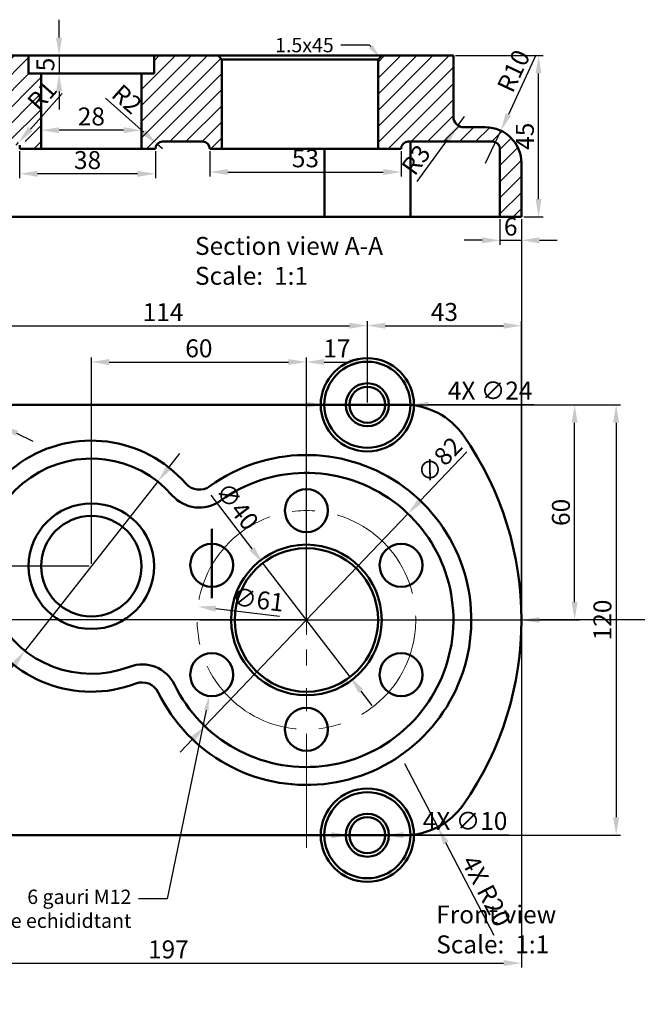
# Model space of a CAD drawing. Units: millimetres. Extents: x 2983 to 3450, y 1738 to 2029.
# Tile 2 of 3: x 3108 to 3281, y 1738 to 2013. Entities that reach past the tile are written whole.
import ezdxf
from ezdxf import colors
from ezdxf.entities.mleader import LeaderData, LeaderLine
from ezdxf.math import Vec2, Vec3

# ---------------------------------------------------------------- set-up
doc = ezdxf.new("R2010")
doc.units = ezdxf.units.MM
doc.linetypes.add('CENTER', pattern=[50.8, 31.75, -6.35, 6.35, -6.35])
for name, color, linetype, lineweight in [('M-CNTR', 1, 'CENTER', 18), ('M-DIMS', 2, 'Continuous', 25), ('M-HATC', 8, 'Continuous', 18), ('M-OUTL', 7, 'Continuous', 50), ('M-TEXT', 3, 'Continuous', 25)]:
    doc.layers.add(name, color=color, linetype=linetype, lineweight=lineweight)
doc.styles.get("Standard").update_dxf_attribs({"font": 'arial.ttf'})
doc.dimstyles.new('ISO-25', dxfattribs={"dimtxt": 5, "dimasz": 5, "dimexe": 1.25, "dimexo": 0.625, "dimtad": 1, "dimdec": 0, "dimtxsty": 'Standard', "dimcen": 2.5, "dimadec": 0, "dimazin": 0, "dimtfac": 1, "dimtdec": 0, "dimtmove": 0, "dimatfit": 3, "dimfxl": 1, "dimarcsym": 0})

# ---------------------------------------------------------------- blocks, each defined once
blk = doc.blocks.new('*U1')
blk.add_circle((0, 0), 6)
blk = doc.blocks.new('*U2')
at = {"layer": 'M-OUTL', "color": 0, "linetype": 'ByBlock', "lineweight": -2, "transparency": 16777216}
blk.add_blockref('*U1', (3188.47, 1875.81), dxfattribs=at)
for p, rotation in [((3162.06, 1860.56), 59.99999999999999), ((3214.89, 1860.56), 300), ((3162.06, 1830.06), 120), ((3214.89, 1830.06), 240), ((3188.47, 1814.81), 180)]:
    blk.add_blockref('*U1', p, dxfattribs=dict(at, rotation=rotation))
blk = doc.blocks.new('*U3')
at = {"layer": 'M-CNTR', "color": 0, "transparency": 16777216}
for p, q in [((0, 8.2), (0, 63.5)), ((-44.5, 0), (-8.2, 0)), ((8.2, 0), (63.5, 0)), ((0, -63.5), (0, -8.2))]:
    blk.add_line(p, q, dxfattribs=at)
at = {"layer": 'M-CNTR', "color": 0, "linetype": 'Continuous', "transparency": 16777216}
for p, q in [((0, -4.1), (0, 4.1)), ((-4.1, 0), (4.1, 0))]:
    blk.add_line(p, q, dxfattribs=at)
blk = doc.blocks.new('*D4')
at = {"layer": 'Defpoints', "color": 0, "transparency": 16777216}
for p in [(3205.47, 1927.36), (3091.47, 1905.31), (3205.47, 1905.31)]:
    blk.add_point(p, dxfattribs=at)
at = {"layer": 'M-DIMS', "color": 0, "lineweight": -2, "transparency": 16777216}
for p, q in [((3091.47, 1905.94), (3091.47, 1928.61)), ((3096.47, 1927.36), (3200.47, 1927.36)), ((3205.47, 1905.94), (3205.47, 1928.61))]:
    blk.add_line(p, q, dxfattribs=at)
at = {"layer": 'M-DIMS', "color": 0, "transparency": 16777216}
for points in [[(3096.47, 1928.19), (3096.47, 1926.52), (3091.47, 1927.36)], [(3200.47, 1928.19), (3200.47, 1926.52), (3205.47, 1927.36)]]:
    blk.add_solid(points, dxfattribs=at)
at = {"layer": 'M-DIMS', "color": 0, "transparency": 16777216, "insert": (3148.47, 1930.49), "char_height": 5, "attachment_point": 5}
blk.add_mtext('114', dxfattribs=at)
blk = doc.blocks.new('*D5')
at = {"layer": 'Defpoints', "color": 0, "transparency": 16777216}
for p in [(3188.47, 1917.23), (3128.47, 1860.31), (3188.47, 1845.31)]:
    blk.add_point(p, dxfattribs=at)
at = {"layer": 'M-DIMS', "color": 0, "lineweight": -2, "transparency": 16777216}
for p, q in [((3128.47, 1860.94), (3128.47, 1918.48)), ((3133.47, 1917.23), (3183.47, 1917.23)), ((3188.47, 1845.94), (3188.47, 1918.48))]:
    blk.add_line(p, q, dxfattribs=at)
at = {"layer": 'M-DIMS', "color": 0, "transparency": 16777216}
for points in [[(3133.47, 1918.07), (3133.47, 1916.4), (3128.47, 1917.23)], [(3183.47, 1918.07), (3183.47, 1916.4), (3188.47, 1917.23)]]:
    blk.add_solid(points, dxfattribs=at)
at = {"layer": 'M-DIMS', "color": 0, "transparency": 16777216, "insert": (3158.47, 1920.41), "char_height": 5, "attachment_point": 5}
blk.add_mtext('60', dxfattribs=at)
blk = doc.blocks.new('*D6')
at = {"layer": 'Defpoints', "color": 0, "transparency": 16777216}
for p in [(3205.47, 1917.23), (3205.47, 1905.31), (3188.47, 1845.31)]:
    blk.add_point(p, dxfattribs=at)
at = {"layer": 'M-DIMS', "color": 0, "lineweight": -2, "transparency": 16777216}
for p, q in [((3188.47, 1845.94), (3188.47, 1918.48)), ((3193.47, 1917.23), (3200.47, 1917.23)), ((3205.47, 1905.94), (3205.47, 1918.48))]:
    blk.add_line(p, q, dxfattribs=at)
at = {"layer": 'M-DIMS', "color": 0, "transparency": 16777216}
for points in [[(3193.47, 1918.07), (3193.47, 1916.4), (3188.47, 1917.23)], [(3200.47, 1918.07), (3200.47, 1916.4), (3205.47, 1917.23)]]:
    blk.add_solid(points, dxfattribs=at)
at = {"layer": 'M-DIMS', "color": 0, "transparency": 16777216, "insert": (3196.97, 1920.37), "char_height": 5, "attachment_point": 5}
blk.add_mtext('17', dxfattribs=at)
blk = doc.blocks.new('*D7')
at = {"layer": 'Defpoints', "color": 0, "transparency": 16777216}
for p in [(3248.47, 1927.36), (3205.47, 1905.31), (3248.47, 1845.31)]:
    blk.add_point(p, dxfattribs=at)
at = {"layer": 'M-DIMS', "color": 0, "lineweight": -2, "transparency": 16777216}
for p, q in [((3205.47, 1905.94), (3205.47, 1928.61)), ((3210.47, 1927.36), (3243.47, 1927.36)), ((3248.47, 1845.94), (3248.47, 1928.61))]:
    blk.add_line(p, q, dxfattribs=at)
at = {"layer": 'M-DIMS', "color": 0, "transparency": 16777216}
for points in [[(3210.47, 1928.19), (3210.47, 1926.52), (3205.47, 1927.36)], [(3243.47, 1928.19), (3243.47, 1926.52), (3248.47, 1927.36)]]:
    blk.add_solid(points, dxfattribs=at)
at = {"layer": 'M-DIMS', "color": 0, "transparency": 16777216, "insert": (3226.97, 1930.54), "char_height": 5, "attachment_point": 5}
blk.add_mtext('43', dxfattribs=at)
blk = doc.blocks.new('*D8')
at = {"layer": 'Defpoints', "color": 0, "transparency": 16777216}
for p in [(3218.47, 1905.31), (3263.3, 1905.31), (3248.47, 1845.31)]:
    blk.add_point(p, dxfattribs=at)
at = {"layer": 'M-DIMS', "color": 0, "lineweight": -2, "transparency": 16777216}
for p, q in [((3219.1, 1905.31), (3264.55, 1905.31)), ((3263.3, 1850.31), (3263.3, 1900.31)), ((3249.1, 1845.31), (3264.55, 1845.31))]:
    blk.add_line(p, q, dxfattribs=at)
at = {"layer": 'M-DIMS', "color": 0, "transparency": 16777216}
for points in [[(3262.47, 1900.31), (3264.13, 1900.31), (3263.3, 1905.31)], [(3262.47, 1850.31), (3264.13, 1850.31), (3263.3, 1845.31)]]:
    blk.add_solid(points, dxfattribs=at)
at = {"layer": 'M-DIMS', "color": 0, "transparency": 16777216, "insert": (3260.12, 1875.31), "char_height": 5, "attachment_point": 5, "rotation": 90}
blk.add_mtext('60', dxfattribs=at)
blk = doc.blocks.new('*D9')
at = {"layer": 'Defpoints', "color": 0, "transparency": 16777216}
for p in [(3205.47, 1905.31), (3205.47, 1785.31), (3274.88, 1785.31)]:
    blk.add_point(p, dxfattribs=at)
at = {"layer": 'M-DIMS', "color": 0, "lineweight": -2, "transparency": 16777216}
for p, q in [((3206.1, 1905.31), (3276.13, 1905.31)), ((3274.88, 1900.31), (3274.88, 1790.31)), ((3206.1, 1785.31), (3276.13, 1785.31))]:
    blk.add_line(p, q, dxfattribs=at)
at = {"layer": 'M-DIMS', "color": 0, "transparency": 16777216}
for points in [[(3274.04, 1900.31), (3275.71, 1900.31), (3274.88, 1905.31)], [(3274.04, 1790.31), (3275.71, 1790.31), (3274.88, 1785.31)]]:
    blk.add_solid(points, dxfattribs=at)
at = {"layer": 'M-DIMS', "color": 0, "transparency": 16777216, "insert": (3271.7, 1845.31), "char_height": 5, "attachment_point": 5, "rotation": 90}
blk.add_mtext('120', dxfattribs=at)
blk = doc.blocks.new('*D10')
at = {"layer": 'Defpoints', "color": 0, "transparency": 16777216}
for p in [(3084.47, 1860.31), (3128.47, 1860.31), (3188.47, 1845.31)]:
    blk.add_point(p, dxfattribs=at)
at = {"layer": 'M-DIMS', "color": 0, "lineweight": -2, "transparency": 16777216}
for p, q in [((3127.85, 1860.31), (3083.22, 1860.31)), ((3084.47, 1850.31), (3084.47, 1855.31)), ((3187.85, 1845.31), (3083.22, 1845.31))]:
    blk.add_line(p, q, dxfattribs=at)
at = {"layer": 'M-DIMS', "color": 0, "transparency": 16777216}
for points in [[(3083.64, 1855.31), (3085.3, 1855.31), (3084.47, 1860.31)], [(3083.64, 1850.31), (3085.3, 1850.31), (3084.47, 1845.31)]]:
    blk.add_solid(points, dxfattribs=at)
at = {"layer": 'M-DIMS', "color": 0, "transparency": 16777216, "insert": (3081.29, 1852.81), "char_height": 5, "attachment_point": 5, "rotation": 90}
blk.add_mtext('15', dxfattribs=at)
blk = doc.blocks.new('*D11')
at = {"layer": 'Defpoints', "color": 0, "transparency": 16777216}
for p in [(3079.81, 1911.05), (3103.14, 1899.57)]:
    blk.add_point(p, dxfattribs=at)
at = {"layer": 'M-DIMS', "color": 0, "lineweight": -2, "transparency": 16777216}
for p, q in [((3058.41, 1921.58), (3075.32, 1913.26)), ((3103.14, 1899.57), (3079.81, 1911.05)), ((3107.63, 1897.37), (3112.11, 1895.16))]:
    blk.add_line(p, q, dxfattribs=at)
at = {"layer": 'M-DIMS', "color": 0, "transparency": 16777216}
for points in [[(3075.69, 1914.01), (3074.96, 1912.51), (3079.81, 1911.05)], [(3107.99, 1898.11), (3107.26, 1896.62), (3103.14, 1899.57)]]:
    blk.add_solid(points, dxfattribs=at)
at = {"layer": 'M-DIMS', "color": 0, "transparency": 16777216, "insert": (3066.09, 1921.5), "char_height": 5, "attachment_point": 5, "rotation": 333.8021}
blk.add_mtext('∅26', dxfattribs=at)
blk = doc.blocks.new('*D12')
at = {"layer": 'Defpoints', "color": 0, "transparency": 16777216}
for p in [(3176.31, 1861.19), (3200.64, 1829.44)]:
    blk.add_point(p, dxfattribs=at)
at = {"layer": 'M-DIMS', "color": 0, "lineweight": -2, "transparency": 16777216}
for p, q in [((3161.81, 1880.1), (3173.27, 1865.15)), ((3200.64, 1829.44), (3176.31, 1861.19)), ((3203.68, 1825.47), (3206.72, 1821.5))]:
    blk.add_line(p, q, dxfattribs=at)
at = {"layer": 'M-DIMS', "color": 0, "transparency": 16777216}
for points in [[(3173.93, 1865.66), (3172.61, 1864.65), (3176.31, 1861.19)], [(3204.34, 1825.98), (3203.02, 1824.96), (3200.64, 1829.44)]]:
    blk.add_solid(points, dxfattribs=at)
at = {"layer": 'M-DIMS', "color": 0, "transparency": 16777216, "insert": (3168.65, 1876.63), "char_height": 5, "attachment_point": 5, "rotation": 307.4676}
blk.add_mtext('∅40', dxfattribs=at)
blk = doc.blocks.new('*D13')
at = {"layer": 'Defpoints', "color": 0, "transparency": 16777216}
for p in [(3158.21, 1849.06), (3218.74, 1841.56)]:
    blk.add_point(p, dxfattribs=at)
at = {"layer": 'M-DIMS', "color": 0, "lineweight": -2, "transparency": 16777216}
blk.add_line((3180.92, 1846.25), (3163.17, 1848.45), dxfattribs=at)
at = {"layer": 'M-DIMS', "color": 0, "transparency": 16777216}
blk.add_solid([(3163.27, 1849.27), (3163.07, 1847.62), (3158.21, 1849.06)], dxfattribs=at)
at = {"layer": 'M-DIMS', "color": 0, "transparency": 16777216, "insert": (3174.93, 1850.33), "char_height": 5, "attachment_point": 5, "rotation": 352.9363}
blk.add_mtext('∅61', dxfattribs=at)
blk = doc.blocks.new('*D14')
at = {"layer": 'Defpoints', "color": 0, "transparency": 16777216}
for p in [(3147.01, 1883.9), (3109.94, 1836.72)]:
    blk.add_point(p, dxfattribs=at)
at = {"layer": 'M-DIMS', "color": 0, "lineweight": -2, "transparency": 16777216}
for p, q in [((3150.09, 1887.84), (3153.18, 1891.77)), ((3147.01, 1883.9), (3109.94, 1836.72)), ((3095.22, 1817.98), (3106.85, 1832.79))]:
    blk.add_line(p, q, dxfattribs=at)
at = {"layer": 'M-DIMS', "color": 0, "transparency": 16777216}
for points in [[(3149.44, 1888.35), (3150.75, 1887.32), (3147.01, 1883.9)], [(3106.2, 1833.3), (3107.51, 1832.27), (3109.94, 1836.72)]]:
    blk.add_solid(points, dxfattribs=at)
at = {"layer": 'M-DIMS', "color": 0, "transparency": 16777216, "insert": (3096.88, 1825.47), "char_height": 5, "attachment_point": 5, "rotation": 51.8501}
blk.add_mtext('∅60', dxfattribs=at)
blk = doc.blocks.new('*D15')
at = {"layer": 'Defpoints', "color": 0, "transparency": 16777216}
for p in [(3216.8, 1874.95), (3160.15, 1815.67)]:
    blk.add_point(p, dxfattribs=at)
at = {"layer": 'M-DIMS', "color": 0, "lineweight": -2, "transparency": 16777216}
for p, q in [((3233.24, 1892.16), (3220.25, 1878.57)), ((3160.15, 1815.67), (3216.8, 1874.95)), ((3156.7, 1812.05), (3153.24, 1808.44))]:
    blk.add_line(p, q, dxfattribs=at)
at = {"layer": 'M-DIMS', "color": 0, "transparency": 16777216}
for points in [[(3219.65, 1879.14), (3220.86, 1877.99), (3216.8, 1874.95)], [(3156.09, 1812.63), (3157.3, 1811.48), (3160.15, 1815.67)]]:
    blk.add_solid(points, dxfattribs=at)
at = {"layer": 'M-DIMS', "color": 0, "transparency": 16777216, "insert": (3226.08, 1889.47), "char_height": 5, "attachment_point": 5, "rotation": 46.3017}
blk.add_mtext('∅82', dxfattribs=at)
blk = doc.blocks.new('*D16')
at = {"layer": 'Defpoints', "color": 0, "transparency": 16777216}
for p in [(3110.97, 2002.67), (3110.97, 1997.67), (3119.46, 1997.67)]:
    blk.add_point(p, dxfattribs=at)
at = {"layer": 'M-DIMS', "color": 0, "lineweight": -2, "transparency": 16777216}
for p, q in [((3119.46, 2007.67), (3119.46, 2012.67)), ((3111.6, 2002.67), (3120.71, 2002.67)), ((3119.46, 2002.67), (3119.46, 1997.67)), ((3111.6, 1997.67), (3120.71, 1997.67)), ((3119.46, 1992.67), (3119.46, 1987.67))]:
    blk.add_line(p, q, dxfattribs=at)
at = {"layer": 'M-DIMS', "color": 0, "transparency": 16777216}
for points in [[(3118.63, 2007.67), (3120.3, 2007.67), (3119.46, 2002.67)], [(3118.63, 1992.67), (3120.3, 1992.67), (3119.46, 1997.67)]]:
    blk.add_solid(points, dxfattribs=at)
at = {"layer": 'M-DIMS', "color": 0, "transparency": 16777216, "insert": (3116.29, 2000.17), "char_height": 5, "attachment_point": 5, "rotation": 90}
blk.add_mtext('5', dxfattribs=at)
blk = doc.blocks.new('*D17')
at = {"layer": 'Defpoints', "color": 0, "transparency": 16777216}
for p in [(3114.47, 1981.87), (3114.47, 1976.67), (3142.47, 1976.67)]:
    blk.add_point(p, dxfattribs=at)
at = {"layer": 'M-DIMS', "color": 0, "lineweight": -2, "transparency": 16777216}
for p, q in [((3114.47, 1977.3), (3114.47, 1983.12)), ((3142.47, 1977.3), (3142.47, 1983.12)), ((3137.47, 1981.87), (3119.47, 1981.87))]:
    blk.add_line(p, q, dxfattribs=at)
at = {"layer": 'M-DIMS', "color": 0, "transparency": 16777216}
for points in [[(3119.47, 1982.7), (3119.47, 1981.03), (3114.47, 1981.87)], [(3137.47, 1982.7), (3137.47, 1981.03), (3142.47, 1981.87)]]:
    blk.add_solid(points, dxfattribs=at)
at = {"layer": 'M-DIMS', "color": 0, "transparency": 16777216, "insert": (3128.47, 1985.05), "char_height": 5, "attachment_point": 5}
blk.add_mtext('28', dxfattribs=at)
blk = doc.blocks.new('*D18')
at = {"layer": 'Defpoints', "color": 0, "transparency": 16777216}
for p in [(3108.47, 1976.67), (3146.34, 1976.67), (3108.47, 1969.71)]:
    blk.add_point(p, dxfattribs=at)
at = {"layer": 'M-DIMS', "color": 0, "lineweight": -2, "transparency": 16777216}
for p, q in [((3108.47, 1976.05), (3108.47, 1968.46)), ((3146.34, 1976.05), (3146.34, 1968.46)), ((3141.34, 1969.71), (3113.47, 1969.71))]:
    blk.add_line(p, q, dxfattribs=at)
at = {"layer": 'M-DIMS', "color": 0, "transparency": 16777216}
for points in [[(3113.47, 1970.54), (3113.47, 1968.87), (3108.47, 1969.71)], [(3141.34, 1970.54), (3141.34, 1968.87), (3146.34, 1969.71)]]:
    blk.add_solid(points, dxfattribs=at)
at = {"layer": 'M-DIMS', "color": 0, "transparency": 16777216, "insert": (3127.41, 1972.89), "char_height": 5, "attachment_point": 5}
blk.add_mtext('38', dxfattribs=at)
blk = doc.blocks.new('*D19')
at = {"layer": 'Defpoints', "color": 0, "transparency": 16777216}
for p in [(3161.52, 1976.67), (3214.89, 1976.67), (3214.89, 1970.2)]:
    blk.add_point(p, dxfattribs=at)
at = {"layer": 'M-DIMS', "color": 0, "lineweight": -2, "transparency": 16777216}
for p, q in [((3161.52, 1976.05), (3161.52, 1968.95)), ((3214.89, 1976.05), (3214.89, 1968.95)), ((3166.52, 1970.2), (3209.89, 1970.2))]:
    blk.add_line(p, q, dxfattribs=at)
at = {"layer": 'M-DIMS', "color": 0, "transparency": 16777216}
for points in [[(3166.52, 1971.04), (3166.52, 1969.37), (3161.52, 1970.2)], [(3209.89, 1971.04), (3209.89, 1969.37), (3214.89, 1970.2)]]:
    blk.add_solid(points, dxfattribs=at)
at = {"layer": 'M-DIMS', "color": 0, "transparency": 16777216, "insert": (3188.2, 1973.38), "char_height": 5, "attachment_point": 5}
blk.add_mtext('53', dxfattribs=at)
blk = doc.blocks.new('*D20')
at = {"layer": 'Defpoints', "color": 0, "transparency": 16777216}
for p in [(3242.47, 1957.67), (3248.47, 1957.67), (3248.47, 1951.16)]:
    blk.add_point(p, dxfattribs=at)
at = {"layer": 'M-DIMS', "color": 0, "lineweight": -2, "transparency": 16777216}
for p, q in [((3242.47, 1957.05), (3242.47, 1949.91)), ((3248.47, 1957.05), (3248.47, 1949.91)), ((3237.47, 1951.16), (3232.47, 1951.16)), ((3242.47, 1951.16), (3248.47, 1951.16)), ((3253.47, 1951.16), (3258.47, 1951.16))]:
    blk.add_line(p, q, dxfattribs=at)
at = {"layer": 'M-DIMS', "color": 0, "transparency": 16777216}
for points in [[(3237.47, 1952), (3237.47, 1950.33), (3242.47, 1951.16)], [(3253.47, 1952), (3253.47, 1950.33), (3248.47, 1951.16)]]:
    blk.add_solid(points, dxfattribs=at)
at = {"layer": 'M-DIMS', "color": 0, "transparency": 16777216, "insert": (3245.47, 1954.34), "char_height": 5, "attachment_point": 5}
blk.add_mtext('6', dxfattribs=at)
blk = doc.blocks.new('*D21')
at = {"layer": 'Defpoints', "color": 0, "transparency": 16777216}
for p in [(3229.47, 2002.67), (3253.24, 2002.67), (3248.47, 1957.67)]:
    blk.add_point(p, dxfattribs=at)
at = {"layer": 'M-DIMS', "color": 0, "lineweight": -2, "transparency": 16777216}
for p, q in [((3230.1, 2002.67), (3254.49, 2002.67)), ((3253.24, 1962.67), (3253.24, 1997.67)), ((3249.1, 1957.67), (3254.49, 1957.67))]:
    blk.add_line(p, q, dxfattribs=at)
at = {"layer": 'M-DIMS', "color": 0, "transparency": 16777216}
for points in [[(3252.4, 1997.67), (3254.07, 1997.67), (3253.24, 2002.67)], [(3252.4, 1962.67), (3254.07, 1962.67), (3253.24, 1957.67)]]:
    blk.add_solid(points, dxfattribs=at)
at = {"layer": 'M-DIMS', "color": 0, "transparency": 16777216, "insert": (3250.07, 1980.17), "char_height": 5, "attachment_point": 5, "rotation": 90}
blk.add_mtext('45', dxfattribs=at)
blk = doc.blocks.new('*D22')
at = {"layer": 'Defpoints', "color": 0, "transparency": 16777216}
for p in [(3232.47, 1985.67), (3230.72, 1983.24)]:
    blk.add_point(p, dxfattribs=at)
at = {"layer": 'M-DIMS', "color": 0, "lineweight": -2, "transparency": 16777216}
for p, q in [((3232.47, 1985.67), (3230.72, 1983.24)), ((3219.41, 1967.58), (3227.79, 1979.19))]:
    blk.add_line(p, q, dxfattribs=at)
at = {"layer": 'M-DIMS', "color": 0, "transparency": 16777216}
blk.add_solid([(3227.12, 1979.67), (3228.47, 1978.7), (3230.72, 1983.24)], dxfattribs=at)
at = {"layer": 'M-DIMS', "color": 0, "transparency": 16777216, "insert": (3219.56, 1973.22), "char_height": 5, "attachment_point": 5, "rotation": 54.1689}
blk.add_mtext('R3', dxfattribs=at)
blk = doc.blocks.new('*D23')
at = {"layer": 'Defpoints', "color": 0, "transparency": 16777216}
for p in [(3242.71, 1981.73), (3238.47, 1972.67)]:
    blk.add_point(p, dxfattribs=at)
at = {"layer": 'M-DIMS', "color": 0, "lineweight": -2, "transparency": 16777216}
for p, q in [((3252.51, 2002.74), (3244.82, 1986.26)), ((3238.47, 1972.67), (3242.71, 1981.73))]:
    blk.add_line(p, q, dxfattribs=at)
at = {"layer": 'M-DIMS', "color": 0, "transparency": 16777216}
blk.add_solid([(3244.07, 1986.61), (3245.58, 1985.91), (3242.71, 1981.73)], dxfattribs=at)
at = {"layer": 'M-DIMS', "color": 0, "transparency": 16777216, "insert": (3246.85, 1998.11), "char_height": 5, "attachment_point": 5, "rotation": 64.9678}
blk.add_mtext('R10', dxfattribs=at)
blk = doc.blocks.new('*D24')
at = {"layer": 'Defpoints', "color": 0, "transparency": 16777216}
for p in [(3146.84, 1978), (3148.34, 1976.67)]:
    blk.add_point(p, dxfattribs=at)
at = {"layer": 'M-DIMS', "color": 0, "lineweight": -2, "transparency": 16777216}
for p, q in [((3132.43, 1990.77), (3143.1, 1981.31)), ((3148.34, 1976.67), (3146.84, 1978))]:
    blk.add_line(p, q, dxfattribs=at)
at = {"layer": 'M-DIMS', "color": 0, "transparency": 16777216}
blk.add_solid([(3143.65, 1981.94), (3142.55, 1980.69), (3146.84, 1978)], dxfattribs=at)
at = {"layer": 'M-DIMS', "color": 0, "transparency": 16777216, "insert": (3137.97, 1990.05), "char_height": 5, "attachment_point": 5, "rotation": 318.4482}
blk.add_mtext('R2', dxfattribs=at)
blk = doc.blocks.new('CBORE-HOLE')
for radius in [13, 12, 6, 5]:
    blk.add_circle((3205.47, 1905.31), radius)
blk = doc.blocks.new('*D36')
at = {"layer": 'Defpoints', "color": 0, "transparency": 16777216}
for p in [(3051.47, 1957.67), (3248.47, 1957.67), (3248.47, 1749.65)]:
    blk.add_point(p, dxfattribs=at)
at = {"layer": 'M-DIMS', "color": 0, "lineweight": -2, "transparency": 16777216}
for p, q in [((3051.47, 1957.05), (3051.47, 1748.4)), ((3248.47, 1957.05), (3248.47, 1748.4)), ((3056.47, 1749.65), (3243.47, 1749.65))]:
    blk.add_line(p, q, dxfattribs=at)
at = {"layer": 'M-DIMS', "color": 0, "transparency": 16777216}
for points in [[(3056.47, 1750.48), (3056.47, 1748.81), (3051.47, 1749.65)], [(3243.47, 1750.48), (3243.47, 1748.81), (3248.47, 1749.65)]]:
    blk.add_solid(points, dxfattribs=at)
at = {"layer": 'M-DIMS', "color": 0, "transparency": 16777216, "insert": (3149.97, 1752.82), "char_height": 5, "attachment_point": 5}
blk.add_mtext('197', dxfattribs=at)
blk = doc.blocks.new('*D39')
at = {"layer": 'Defpoints', "color": 0, "transparency": 16777216}
for p in [(3193.47, 1905.31), (3217.47, 1905.31)]:
    blk.add_point(p, dxfattribs=at)
at = {"layer": 'M-DIMS', "color": 0, "lineweight": -2, "transparency": 16777216}
for p, q in [((3188.47, 1905.31), (3183.47, 1905.31)), ((3193.47, 1905.31), (3217.47, 1905.31)), ((3251.99, 1905.31), (3222.47, 1905.31))]:
    blk.add_line(p, q, dxfattribs=at)
at = {"layer": 'M-DIMS', "color": 0, "transparency": 16777216}
for points in [[(3188.47, 1906.14), (3188.47, 1904.48), (3193.47, 1905.31)], [(3222.47, 1906.15), (3222.47, 1904.48), (3217.47, 1905.31)]]:
    blk.add_solid(points, dxfattribs=at)
at = {"layer": 'M-DIMS', "color": 0, "transparency": 16777216, "insert": (3239.73, 1908.63), "char_height": 5, "attachment_point": 5, "rotation": 0.0019}
blk.add_mtext('4X ∅24', dxfattribs=at)
blk = doc.blocks.new('*D41')
at = {"layer": 'Defpoints', "color": 0, "transparency": 16777216}
for p in [(3200.47, 1785.31), (3210.47, 1785.31)]:
    blk.add_point(p, dxfattribs=at)
at = {"layer": 'M-DIMS', "color": 0, "lineweight": -2, "transparency": 16777216}
for p, q in [((3195.47, 1785.31), (3190.47, 1785.31)), ((3200.47, 1785.31), (3210.47, 1785.31)), ((3244.99, 1785.31), (3215.47, 1785.31))]:
    blk.add_line(p, q, dxfattribs=at)
at = {"layer": 'M-DIMS', "color": 0, "transparency": 16777216}
for points in [[(3195.47, 1786.14), (3195.47, 1784.48), (3200.47, 1785.31)], [(3215.47, 1786.15), (3215.47, 1784.48), (3210.47, 1785.31)]]:
    blk.add_solid(points, dxfattribs=at)
at = {"layer": 'M-DIMS', "color": 0, "transparency": 16777216, "insert": (3232.73, 1788.63), "char_height": 5, "attachment_point": 5, "rotation": 0.0047}
blk.add_mtext('4X ∅10', dxfattribs=at)
blk = doc.blocks.new('*D42')
at = {"layer": 'Defpoints', "color": 0, "transparency": 16777216}
for p in [(3051.47, 1845.31), (3151.47, 1845.31)]:
    blk.add_point(p, dxfattribs=at)
at = {"layer": 'M-DIMS', "color": 0, "lineweight": -2, "transparency": 16777216}
for p, q in [((2982.94, 1845.31), (3046.47, 1845.31)), ((3151.47, 1845.31), (3051.47, 1845.31))]:
    blk.add_line(p, q, dxfattribs=at)
at = {"layer": 'M-DIMS', "color": 0, "transparency": 16777216}
blk.add_solid([(3046.47, 1846.15), (3046.47, 1844.48), (3051.47, 1845.31)], dxfattribs=at)
at = {"layer": 'M-DIMS', "color": 0, "transparency": 16777216, "insert": (2991.47, 1848.49), "char_height": 5, "attachment_point": 5, "rotation": 359.9998}
blk.add_mtext('R100', dxfattribs=at)
blk = doc.blocks.new('*D43')
at = {"layer": 'Defpoints', "color": 0, "transparency": 16777216}
for p in [(3158.71, 1845.31), (3248.47, 1845.31)]:
    blk.add_point(p, dxfattribs=at)
at = {"layer": 'M-DIMS', "color": 0, "lineweight": -2, "transparency": 16777216}
for p, q in [((3158.71, 1845.31), (3248.47, 1845.31)), ((3313.78, 1845.31), (3253.47, 1845.31))]:
    blk.add_line(p, q, dxfattribs=at)
at = {"layer": 'M-DIMS', "color": 0, "transparency": 16777216}
blk.add_solid([(3253.47, 1846.15), (3253.47, 1844.48), (3248.47, 1845.31)], dxfattribs=at)
at = {"layer": 'M-DIMS', "color": 0, "transparency": 16777216, "insert": (3302.33, 1848.49), "char_height": 5, "attachment_point": 5, "rotation": 0.0003}
blk.add_mtext('R89.76', dxfattribs=at)
blk = doc.blocks.new('*D44')
at = {"layer": 'Defpoints', "color": 0, "transparency": 16777216}
for p in [(3215.87, 1805.31), (3225.1, 1787.57)]:
    blk.add_point(p, dxfattribs=at)
at = {"layer": 'M-DIMS', "color": 0, "lineweight": -2, "transparency": 16777216}
for p, q in [((3215.87, 1805.31), (3225.1, 1787.57)), ((3240.87, 1757.3), (3227.41, 1783.14))]:
    blk.add_line(p, q, dxfattribs=at)
at = {"layer": 'M-DIMS', "color": 0, "transparency": 16777216}
blk.add_solid([(3228.15, 1783.52), (3226.67, 1782.75), (3225.1, 1787.57)], dxfattribs=at)
at = {"layer": 'M-DIMS', "color": 0, "transparency": 16777216, "insert": (3238.11, 1769.47), "char_height": 5, "attachment_point": 5, "rotation": 297.5065}
blk.add_mtext('4X R20', dxfattribs=at)
blk = doc.blocks.new('*D46')
at = {"layer": 'Defpoints', "color": 0, "transparency": 16777216}
for p in [(3107.47, 1977.67), (3108.14, 1978.42)]:
    blk.add_point(p, dxfattribs=at)
at = {"layer": 'M-DIMS', "color": 0, "lineweight": -2, "transparency": 16777216}
for p, q in [((3120.33, 1992.13), (3111.46, 1982.16)), ((3107.47, 1977.67), (3108.14, 1978.42))]:
    blk.add_line(p, q, dxfattribs=at)
at = {"layer": 'M-DIMS', "color": 0, "transparency": 16777216}
blk.add_solid([(3110.84, 1982.71), (3112.08, 1981.6), (3108.14, 1978.42)], dxfattribs=at)
at = {"layer": 'M-DIMS', "color": 0, "transparency": 16777216, "insert": (3115.21, 1991.1), "char_height": 5, "attachment_point": 5, "rotation": 48.3754}
blk.add_mtext('R1', dxfattribs=at)

msp = doc.modelspace()

# ---------------------------------------------------------------- hatches: boundary and pattern name
at = {"layer": 'M-HATC'}
h = msp.add_hatch(dxfattribs=at)
h.set_pattern_fill('ANSI31', color=256)
h.set_pattern_definition([(45, (0, -22.2306), (-2.245064, 2.245064), [])])
h.paths.add_polyline_path([(3114.475, 1997.671), (3110.975, 1997.671), (3110.975, 2002.671), (3098.475, 2002.671), (3098.475, 1985.65), (3061.528, 1985.846, 0.4157622), (3051.475, 1975.846), (3051.475, 1957.671), (3057.475, 1957.671), (3057.475, 1975.671, -0.4142136), (3060.475, 1978.671), (3079.476, 1978.671), (3103.475, 1978.671), (3110.475, 1978.671, -0.4142136), (3111.475, 1977.671), (3111.475, 1976.671), (3114.475, 1976.671)])
h.paths.add_polyline_path([(3164.888, 2001.611), (3163.828, 2002.671), (3145.975, 2002.671), (3145.975, 1997.671), (3142.475, 1997.671), (3142.475, 1976.671), (3146.337, 1976.671, -0.4142136), (3148.337, 1978.671), (3159.52, 1978.671, -0.4142136), (3161.52, 1976.671), (3164.888, 1976.671), (3164.888, 1978.671)])
h.paths.add_polyline_path([(3216.888, 1978.671), (3240.475, 1978.671, -0.4142136), (3242.475, 1976.671), (3242.475, 1957.671), (3248.475, 1957.671), (3248.475, 1972.671, 0.4142136), (3238.475, 1982.671), (3232.475, 1982.671, -0.4142136), (3229.475, 1985.671), (3229.475, 2002.671), (3209.535, 2002.671), (3208.475, 2001.611), (3208.475, 1976.671), (3214.888, 1976.671, -0.4142136)])

# ---------------------------------------------------------------- linework, layer by layer
at = {"layer": 'M-CNTR'}
msp.add_circle((3188.475, 1845.312), 30.5, dxfattribs=at)
at = {"layer": 'M-OUTL'}
for p, q in [((3110.975, 2002.671), (3098.475, 2002.671)), ((3110.975, 1997.671), (3110.975, 2002.671)), ((3110.975, 2002.671), (3145.975, 2002.671)), ((3168.475, 2002.671), (3145.975, 2002.671)), ((3145.975, 2002.671), (3145.975, 1997.671)), ((3164.888, 2001.611), (3163.828, 2002.671)), ((3164.888, 1978.671), (3164.888, 2001.611)), ((3208.475, 2001.611), (3164.888, 2001.611)), ((3229.475, 2002.671), (3168.475, 2002.671)), ((3208.475, 2001.611), (3209.535, 2002.671)), ((3208.475, 2001.611), (3208.475, 1976.671)), ((3229.475, 1985.671), (3229.475, 2002.671)), ((3114.475, 1997.671), (3110.975, 1997.671)), ((3142.475, 1997.671), (3114.475, 1997.671)), ((3114.475, 1997.671), (3114.475, 1976.671)), ((3145.975, 1997.671), (3142.475, 1997.671)), ((3142.475, 1997.671), (3142.475, 1976.671)), ((3238.475, 1982.671), (3232.475, 1982.671)), ((3108.475, 1977.671), (3108.475, 1976.671)), ((3111.475, 1976.671), (3108.475, 1976.671)), ((3111.475, 1976.671), (3114.475, 1976.671)), ((3146.337, 1976.671), (3114.475, 1976.671)), ((3146.337, 1976.671), (3146.337, 1976.671)), ((3148.337, 1978.671), (3159.52, 1978.671)), ((3164.888, 1976.671), (3161.52, 1976.671)), ((3161.52, 1976.671), (3161.52, 1976.671)), ((3164.888, 1976.671), (3164.888, 1978.671)), ((3214.888, 1976.671), (3164.888, 1976.671)), ((3193.475, 1957.671), (3193.475, 1976.671)), ((3214.888, 1976.671), (3214.888, 1976.671)), ((3240.475, 1978.671), (3216.888, 1978.671)), ((3217.475, 1978.671), (3217.475, 1957.671)), ((3242.475, 1976.671), (3242.475, 1957.671)), ((3248.475, 1957.671), (3248.475, 1972.671)), ((3051.475, 1957.671), (3248.475, 1957.671)), ((3205.475, 1905.312), (3091.475, 1905.312)), ((3205.475, 1905.312), (3215.868, 1905.312)), ((3162.061, 1860.562), (3162.061, 1870.681)), ((3162.061, 1870.681), (3162.061, 1851.412)), ((3091.475, 1785.312), (3205.475, 1785.312)), ((3205.475, 1785.312), (3215.868, 1785.312))]:
    msp.add_line(p, q, dxfattribs=at)
for centre, radius in [((3128.475, 1860.312), 17.5), ((3128.475, 1860.312), 14), ((3188.475, 1845.312), 21), ((3188.475, 1845.312), 20)]:
    msp.add_circle(centre, radius, dxfattribs=at)
for centre, radius, start, end in [((3232.475, 1985.671), 3, 180, 270), ((3238.475, 1972.671), 10, 360, 90), ((3148.337, 1976.671), 2, 90, 180), ((3159.52, 1976.671), 2, 0, 90), ((3216.888, 1976.671), 2, 90, 180), ((3240.475, 1976.671), 2, 0, 90), ((3215.868, 1885.312), 20, 34.98678, 90), ((3128.475, 1860.312), 35, 41.16002, 290.7675), ((3158.714, 1845.312), 89.761, 325.01322, 34.98678), ((3128.475, 1860.312), 30, 41.16002, 290.7675), ((3188.475, 1845.312), 46, 206.0552, 125.87231), ((3188.475, 1845.312), 41, 206.0552, 125.87231), ((3158.59, 1886.638), 5, 221.16002, 305.87231), ((3158.59, 1886.638), 10, 221.16002, 305.87231), ((3142.658, 1822.911), 10, 26.0552, 110.7675), ((3142.658, 1822.911), 5, 26.0552, 110.7675), ((3215.868, 1805.312), 20, 270, 325.01322)]:
    msp.add_arc(centre, radius, start, end, dxfattribs=at)

# ---------------------------------------------------------------- block references
at = {"layer": 'M-CNTR'}
msp.add_blockref('*U3', (3188.475, 1845.312), dxfattribs=at)
at = {"layer": 'M-OUTL'}
for name, p in [('CBORE-HOLE', (0, 0)), ('*U2', (0, 0)), ('CBORE-HOLE', (0, -120))]:
    msp.add_blockref(name, p, dxfattribs=at)

# ---------------------------------------------------------------- texts
at = {"layer": 'M-TEXT', "char_height": 5, "attachment_point": 1}
for s, insert in [('Section view A-A\\PScale:  1:1', (3157.387, 1952.098)), ('Front view\\PScale:  1:1', (3224.688, 1765.7))]:
    msp.add_mtext_dynamic_manual_height_columns(s, width=86.4063, gutter_width=12.5, heights=[0], dxfattribs=dict(at, insert=insert))

# ---------------------------------------------------------------- dimensions: what is measured, and where the dimension line sits
at = {"layer": 'M-DIMS'}
for base, p1, p2, picture, middle in [((3119.462, 1997.671), (3110.975, 2002.671), (3110.975, 1997.671), '*D16', (3116.294, 2000.171)), ((3253.237, 2002.671), (3248.475, 1957.671), (3229.475, 2002.671), '*D21', (3250.07, 1980.171)), ((3274.877, 1785.312), (3205.475, 1905.312), (3205.475, 1785.312), '*D9', (3271.7, 1845.312)), ((3263.299, 1905.312), (3248.475, 1845.312), (3218.475, 1905.312), '*D8', (3260.121, 1875.312)), ((3084.469, 1860.312), (3188.475, 1845.312), (3128.475, 1860.312), '*D10', (3081.291, 1852.812))]:
    dim = msp.add_linear_dim(base=base, p1=p1, p2=p2, angle=90, dimstyle='ISO-25', override={"dimclrd": 0, "dimclre": 0, "dimclrt": 0}, dxfattribs=at)
    dim.commit()
    dim.dimension.update_dxf_attribs({"geometry": picture, "text_midpoint": middle})
for center, mpoint, override, picture, middle in [((3238.475, 1972.671), (3242.706, 1981.732), {"dimclrd": 0, "dimclre": 0, "dimclrt": 0}, '*D23', (3246.846, 1998.108)), ((3107.475, 1977.671), (3108.139, 1978.419), {"dimdec": 0, "dimlfac": 1, "dimrnd": 0, "dimzin": 0, "dimdsep": 46, "dimlunit": 2}, '*D46', (3115.21, 1991.096)), ((3148.337, 1976.671), (3146.84, 1977.998), {"dimclrd": 0, "dimclre": 0, "dimclrt": 0}, '*D24', (3137.971, 1990.049)), ((3232.475, 1985.671), (3230.718, 1983.239), {"dimclrd": 0, "dimclre": 0, "dimclrt": 0}, '*D22', (3219.561, 1973.218))]:
    dim = msp.add_radius_dim(center=center, mpoint=mpoint, dimstyle='ISO-25', override=override, dxfattribs=at)
    dim.commit()
    dim.dimension.update_dxf_attribs({"geometry": picture, "text_midpoint": middle})
for base, p1, p2, override, picture, middle in [((3114.475, 1981.867), (3142.475, 1976.671), (3114.475, 1976.671), {"dimclrd": 0, "dimclre": 0, "dimclrt": 0}, '*D17', (3128.475, 1985.045)), ((3108.475, 1969.706), (3146.337, 1976.671), (3108.475, 1976.671), {"dimclrd": 0, "dimclre": 0, "dimclrt": 0}, '*D18', (3127.406, 1972.885)), ((3214.888, 1970.204), (3161.52, 1976.671), (3214.888, 1976.671), {"dimclrd": 0, "dimclre": 0, "dimclrt": 0}, '*D19', (3188.204, 1973.383)), ((3248.475, 1749.646), (3051.475, 1957.671), (3248.475, 1957.671), {"dimdec": 0, "dimlfac": 1, "dimrnd": 0, "dimzin": 0, "dimdsep": 46, "dimlunit": 2}, '*D36', (3149.975, 1752.824)), ((3248.475, 1951.162), (3242.475, 1957.671), (3248.475, 1957.671), {"dimclrd": 0, "dimclre": 0, "dimclrt": 0}, '*D20', (3245.475, 1954.34)), ((3205.475, 1927.357), (3091.475, 1905.312), (3205.475, 1905.312), {"dimclrd": 0, "dimclre": 0, "dimclrt": 0}, '*D4', (3148.475, 1930.492)), ((3248.475, 1927.357), (3205.475, 1905.312), (3248.475, 1845.312), {"dimclrd": 0, "dimclre": 0, "dimclrt": 0}, '*D7', (3226.975, 1930.537)), ((3188.475, 1917.234), (3128.475, 1860.312), (3188.475, 1845.312), {"dimclrd": 0, "dimclre": 0, "dimclrt": 0}, '*D5', (3158.475, 1920.412)), ((3205.475, 1917.234), (3188.475, 1845.312), (3205.475, 1905.312), {"dimclrd": 0, "dimclre": 0, "dimclrt": 0}, '*D6', (3196.975, 1920.37))]:
    dim = msp.add_linear_dim(base=base, p1=p1, p2=p2, dimstyle='ISO-25', override=override, dxfattribs=at)
    dim.commit()
    dim.dimension.update_dxf_attribs({"geometry": picture, "text_midpoint": middle})
for p1, p2, picture, middle in [((3103.139, 1899.572), (3079.81, 1911.051), '*D11', (3064.624, 1918.522)), ((3160.149, 1815.669), (3216.8, 1874.954), '*D15', (3226.077, 1889.465)), ((3147.006, 1883.904), (3109.943, 1836.72), '*D14', (3096.884, 1825.465)), ((3200.641, 1829.438), (3176.308, 1861.186), '*D12', (3168.65, 1876.631))]:
    dim = msp.add_diameter_dim_2p(p1=p1, p2=p2, dimstyle='ISO-25', override={"dimclrd": 0, "dimclre": 0, "dimclrt": 0}, dxfattribs=at)
    dim.commit()
    dim.dimension.update_dxf_attribs({"geometry": picture, "text_midpoint": middle})
for p1, p2, picture, middle in [((3193.475, 1905.311), (3217.475, 1905.312), '*D39', (3239.73, 1905.313)), ((3200.475, 1785.311), (3210.475, 1785.312), '*D41', (3232.732, 1785.314))]:
    dim = msp.add_diameter_dim_2p(p1=p1, p2=p2, text='4X <>', dimstyle='ISO-25', override={"dimdec": 0, "dimlfac": 1, "dimrnd": 0, "dimzin": 0, "dimdsep": 46, "dimlunit": 2}, dxfattribs=at)
    dim.commit()
    dim.dimension.update_dxf_attribs({"geometry": picture, "text_midpoint": middle, "dimtype": 163})
dim = msp.add_diameter_dim_2p(p1=(3218.743, 1841.561), p2=(3158.206, 1849.062), dimstyle='ISO-25', override={"dimclrd": 0, "dimclre": 0, "dimclrt": 0}, dxfattribs=at)
dim.commit()
dim.dimension.update_dxf_attribs({"geometry": '*D13', "text_midpoint": (3174.525, 1847.04), "dimtype": 163})
for center, mpoint, override, picture, middle in [((3151.475, 1845.312), (3051.475, 1845.312), {"dimdec": 0, "dimlfac": 1, "dimrnd": 0, "dimzin": 0, "dimdsep": 46, "dimlunit": 2}, '*D42', (2991.475, 1845.312)), ((3158.714, 1845.312), (3248.475, 1845.312), {"dimdec": 2, "dimlfac": 1, "dimrnd": 0, "dimzin": 0, "dimdsep": 46, "dimlunit": 2}, '*D43', (3302.331, 1845.312))]:
    dim = msp.add_radius_dim(center=center, mpoint=mpoint, dimstyle='ISO-25', override=override, dxfattribs=at)
    dim.commit()
    dim.dimension.update_dxf_attribs({"geometry": picture, "text_midpoint": middle, "dimtype": 164})
dim = msp.add_radius_dim(center=(3215.868, 1805.312), mpoint=(3225.105, 1787.572), text='4X <>', dimstyle='ISO-25', override={"dimdec": 0, "dimlfac": 1, "dimrnd": 0, "dimzin": 0, "dimdsep": 46, "dimlunit": 2}, dxfattribs=at)
dim.commit()
dim.dimension.update_dxf_attribs({"geometry": '*D44', "text_midpoint": (3238.113, 1769.472)})

# ---------------------------------------------------------------- leaders
ml = msp.add_multileader_mtext('Standard', dxfattribs=at)
ml.set_content('1.5x45', color=256)
ml.set_leader_properties()
ml.build(insert=Vec2(0, 0))
ctx = ml.context
ctx.base_point, ctx.plane_origin = Vec3(3178.145, 2005.553), Vec3(3209.005, 2002.141)
ctx.text_align_type = 2
notes = []
notes.append((ctx, [(0, (1, 1, 0), (3206.09, 2005.553), (-1, 0), 8, [(0, [(3209.005, 2002.141)], 0, [])])]))
ctx.mtext.insert, ctx.mtext.alignment, ctx.mtext.flow_direction = Vec3(3196.09, 2007.587), 3, 5
ml = msp.add_multileader_mtext('Standard', dxfattribs=at)
ml.set_content('6 gauri M12\\Pdiispuse echididtant', color=256)
ml.set_leader_properties()
ml.build(insert=Vec2(0, 0))
ctx = ml.context
ctx.base_point, ctx.plane_origin = Vec3(3088.784, 1767.575), Vec3(3161.337, 1824.105)
ctx.text_align_type = 2
notes.append((ctx, [(0, (1, 1, 0), (3149.635, 1767.575), (-1, 0), 8, [(0, [(3161.337, 1824.105)], 0, [])])]))
ctx.mtext.insert, ctx.mtext.alignment, ctx.mtext.flow_direction = Vec3(3139.635, 1770.13), 3, 5
for ctx, leaders in notes:
    for number, flags, end, landing, length, lines in leaders:
        leader = LeaderData()
        leader.index, (leader.has_last_leader_line, leader.has_dogleg_vector, leader.attachment_direction) = number, flags
        leader.last_leader_point, leader.dogleg_vector, leader.dogleg_length = Vec3(end), Vec3(landing), length
        for number, points, colour, breaks in lines:
            line = LeaderLine()
            line.index, line.vertices, line.color, line.breaks = number, Vec3.list(points), colors.encode_raw_color(colour), breaks
            leader.lines.append(line)
        ctx.leaders.append(leader)

doc.saveas('drawing.dxf')
